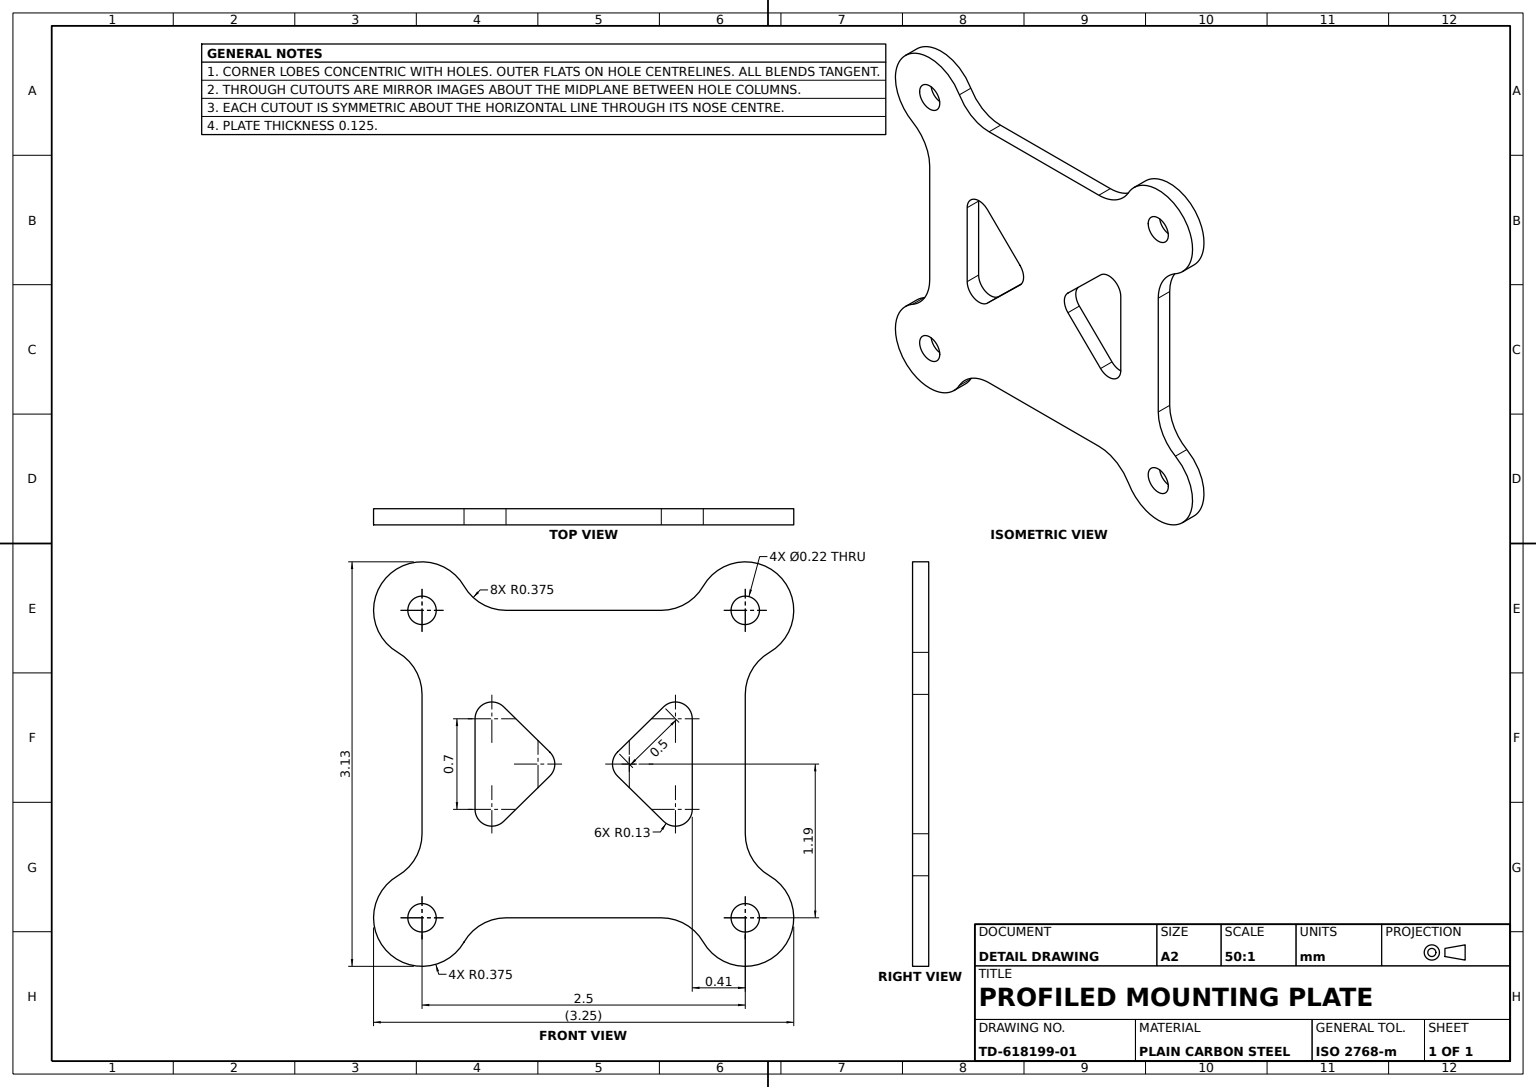
from build123d import *

# Parameters (mm, degrees)
BRACKET_PLATE_PROFILE_R = 0.11
BRACKET_PLATE_DEPTH     = 0.125


with BuildPart() as part:
    # Bracket Plate Profile → Bracket Plate (new body)
    with BuildSketch(Plane.XY):
        with BuildLine():
            Line((-1.25, 0.538480947), (-1.25, -0.538480947))
            ThreePointArc((-1.25, -0.538480947), (-1.300240474, -0.725980947), (-1.4375, -0.863240474))
            ThreePointArc((-1.4375, -0.863240474), (-1.515165043, -1.453165043), (-0.925240474, -1.3755))
            ThreePointArc((-0.925240474, -1.3755), (-0.787980947, -1.238240474), (-0.600480947, -1.188))
            Line((-0.600480947, -1.188), (0.600480947, -1.188))
            ThreePointArc((0.600480947, -1.188), (0.787980947, -1.238240474), (0.925240474, -1.3755))
            ThreePointArc((0.925240474, -1.3755), (1.515165043, -1.453165043), (1.4375, -0.863240474))
            ThreePointArc((1.4375, -0.863240474), (1.300240474, -0.725980947), (1.25, -0.538480947))
            Line((1.25, -0.538480947), (1.25, 0.538480947))
            ThreePointArc((1.25, 0.538480947), (1.300240474, 0.725980947), (1.4375, 0.863240474))
            ThreePointArc((1.4375, 0.863240474), (1.515165043, 1.453165043), (0.925240474, 1.3755))
            ThreePointArc((0.925240474, 1.3755), (0.787980947, 1.238240474), (0.600480947, 1.188))
            Line((0.600480947, 1.188), (-0.600480947, 1.188))
            ThreePointArc((-0.600480947, 1.188), (-0.787980947, 1.238240474), (-0.925240474, 1.3755))
            ThreePointArc((-0.925240474, 1.3755), (-1.515165043, 1.453165043), (-1.4375, 0.863240474))
            ThreePointArc((-1.4375, 0.863240474), (-1.300240474, 0.725980947), (-1.25, 0.538480947))
        make_face()
        with Locations((-1.25, 1.188)):
            Circle(BRACKET_PLATE_PROFILE_R, mode=Mode.SUBTRACT)
        with Locations((1.25, 1.188)):
            Circle(BRACKET_PLATE_PROFILE_R, mode=Mode.SUBTRACT)
        with Locations((1.25, -1.188)):
            Circle(BRACKET_PLATE_PROFILE_R, mode=Mode.SUBTRACT)
        with Locations((-1.25, -1.188)):
            Circle(BRACKET_PLATE_PROFILE_R, mode=Mode.SUBTRACT)
        with BuildLine():
            Line((-0.84, 0.35), (-0.84, -0.35))
            ThreePointArc((-0.84, -0.35), (-0.760348784, -0.469854078), (-0.619, -0.44283857))
            Line((-0.619, -0.44283857), (-0.261928579, -0.09283857))
            ThreePointArc((-0.261928579, -0.09283857), (-0.222928579, 0), (-0.261928579, 0.09283857))
            Line((-0.261928579, 0.09283857), (-0.619, 0.44283857))
            ThreePointArc((-0.619, 0.44283857), (-0.760348784, 0.469854078), (-0.84, 0.35))
        make_face(mode=Mode.SUBTRACT)
        with BuildLine():
            Line((0.619, -0.44283857), (0.261928579, -0.09283857))
            ThreePointArc((0.261928579, -0.09283857), (0.222928579, 0), (0.261928579, 0.09283857))
            Line((0.261928579, 0.09283857), (0.619, 0.44283857))
            ThreePointArc((0.619, 0.44283857), (0.760348784, 0.469854078), (0.84, 0.35))
            Line((0.84, 0.35), (0.84, -0.35))
            ThreePointArc((0.84, -0.35), (0.760348784, -0.469854078), (0.619, -0.44283857))
        make_face(mode=Mode.SUBTRACT)
    extrude(amount=BRACKET_PLATE_DEPTH)


solid = part.part
